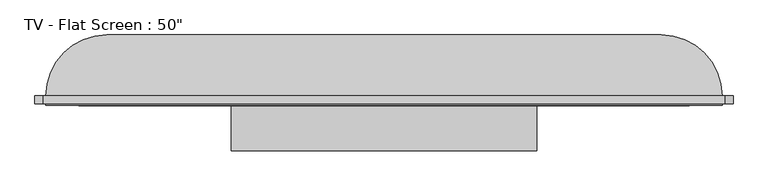
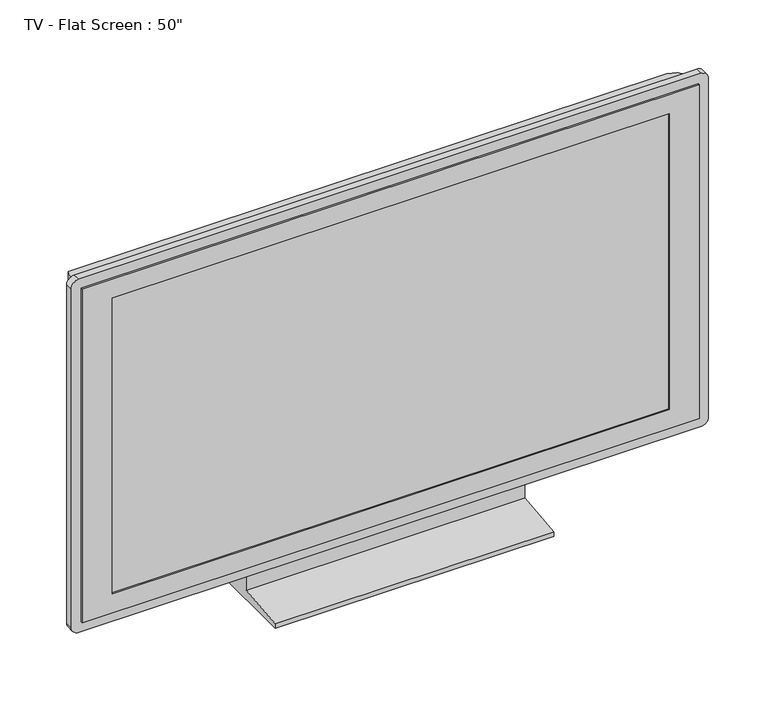
"""IFC4 building model written with IfcOpenShell, lengths in millimetres: furniture geometry."""

from ifc_helpers import new_model, si_unit, point, frame, frame_2d, origin, place, context, project, spatial, polyline, circle_curve, ellipse_curve, trimmed, segment, composite_curve, outline, extrude, faceted_brep, source, transform, mapped, element, save
from ifc_brep_helpers import plane_surface, cylinder_surface, advanced_brep


def furniture_0b81fedb(model_context):
    return source(origin(), model_context, "Body", "SolidModel", [
        advanced_brep(
        [(-617.3827737, -51.4613764, 80.0), (609.4937454, -51.4613764, 80.0), (609.4937454, -51.4613764, 782.6751733), (-617.3827737, -51.4613764, 782.6751733), (499.4937454, 58.5386236, 80.0), (-507.3827737, 58.5386236, 80.0), (-507.3827737, 58.5386236, 672.6751733), (499.4937454, 58.5386236, 672.6751733)],
        [
            (0, 1),
            (1, 2),
            (2, 3),
            (3, 0),
            (4, 5),
            (5, 6),
            (6, 7),
            (7, 4),
            (0, 5, circle_curve(frame((-507.3827737, -51.4613764, 80.0), z_axis=(0.0, 0.0, -1.0), x_axis=(-1.0, 0.0, 0.0)), 110.0)),
            (4, 1, circle_curve(frame((499.4937454, -51.4613764, 80.0), z_axis=(0.0, 0.0, -1.0), x_axis=(1.0, 0.0, 0.0)), 110.0)),
            (7, 2, ellipse_curve(frame((499.4937454, -51.4613764, 672.6751733), z_axis=(0.7071067811865475, 0.0, -0.7071067811865475), x_axis=(0.7071067811865474, 0.0, 0.7071067811865476)), 155.5634919, 110.0)),
            (6, 3, ellipse_curve(frame((-507.3827737, -51.4613764, 672.6751733), z_axis=(0.7071067811865475, 0.0, 0.7071067811865475), x_axis=(-0.7071067811865476, 0.0, 0.7071067811865474)), 155.5634919, 110.0)),
        ],
        [
            plane_surface(frame((-617.3827737, -51.4613764, 782.6751733), z_axis=(0.0, -1.0, 0.0), x_axis=(-1.0, 0.0, 0.0))),
            plane_surface(frame((-617.3827737, 58.5386236, 782.6751733), z_axis=(0.0, 1.0, 0.0), x_axis=(1.0, 0.0, 0.0))),
            plane_surface(frame((-617.3827737, -51.4613764, 80.0), z_axis=(0.0, 0.0, -1.0), x_axis=(0.0, 1.0, 0.0))),
            cylinder_surface(frame((499.4937454, -51.4613764, 80.0), z_axis=(0.0, 0.0, 1.0), x_axis=(1.0, 0.0, 0.0)), 110.0),
            cylinder_surface(frame((609.4937454, -51.4613764, 672.6751733), z_axis=(-1.0, 0.0, 0.0), x_axis=(0.0, 0.0, 1.0)), 110.0),
            cylinder_surface(frame((-507.3827737, -51.4613764, 782.6751733), z_axis=(0.0, 0.0, -1.0), x_axis=(-1.0, 0.0, 0.0)), 110.0),
        ],
        [
            (0, [[1, 2, 3, 4]]),
            (1, [[5, 6, 7, 8]]),
            (2, [[-1, 9, -5, 10]]),
            (3, [[11, -2, -10, -8]]),
            (4, [[-11, -7, 12, -3]]),
            (5, [[-12, -6, -9, -4]]),
        ],
    ),
        extrude(outline(composite_curve([segment(polyline([(802.6751733, 614.4937454), (802.6751733, -622.3827737)]), True, "CONTINUOUS"), segment(trimmed(circle_curve(frame_2d((787.6751733, -622.3827737)), 15.0), [point((802.6751733, -622.3827737))], [point((787.6751733, -637.3827737))], False, "CARTESIAN"), True, "CONTINUOUS"), segment(polyline([(787.6751733, -637.3827737), (75.0, -637.3827737)]), True, "CONTINUOUS"), segment(trimmed(circle_curve(frame_2d((75.0, -622.3827737)), 15.0), [point((75.0, -637.3827737))], [point((60.0, -622.3827737))], False, "CARTESIAN"), True, "CONTINUOUS"), segment(polyline([(60.0, -622.3827737), (60.0, 614.4937454)]), True, "CONTINUOUS"), segment(trimmed(circle_curve(frame_2d((75.0, 614.4937454)), 15.0), [point((60.0, 614.4937454))], [point((75.0, 629.4937454))], False, "CARTESIAN"), True, "CONTINUOUS"), segment(polyline([(75.0, 629.4937454), (787.6751733, 629.4937454)]), True, "CONTINUOUS"), segment(trimmed(circle_curve(frame_2d((787.6751733, 614.4937454)), 15.0), [point((787.6751733, 629.4937454))], [point((802.6751733, 614.4937454))], False, "CARTESIAN"), True, "CONTINUOUS")], self_intersect=False), holes=[polyline([(782.6751733, 609.4937454), (80.0, 609.4937454), (80.0, -617.3827737), (782.6751733, -617.3827737), (782.6751733, 609.4937454)])]), frame((0.0, -66.4613764, 0.0), z_axis=(0.0, 1.0, 0.0), x_axis=(0.0, 0.0, 1.0)), (0.0, 0.0, 1.0), 15.0),
        faceted_brep([(609.4937454, -69.4613764, 782.6751733), (-617.3827737, -69.4613764, 782.6751733), (-617.3827737, -69.4613764, 80.0), (609.4937454, -69.4613764, 80.0), (-557.3827737, -69.4613764, 742.6751733), (549.4937454, -69.4613764, 742.6751733), (549.4937454, -69.4613764, 120.0), (-557.3827737, -69.4613764, 120.0), (609.4937454, -51.4613764, 782.6751733), (609.4937454, -51.4613764, 80.0), (-617.3827737, -51.4613764, 80.0), (-617.3827737, -51.4613764, 782.6751733), (-557.3827737, -66.4613764, 742.6751733), (-557.3827737, -66.4613764, 120.0), (549.4937454, -66.4613764, 120.0), (549.4937454, -66.4613764, 742.6751733)], [[[0, 1, 2, 3], [4, 5, 6, 7]], [[8, 9, 10, 11]], [[1, 0, 8, 11]], [[2, 1, 11, 10]], [[3, 2, 10, 9]], [[0, 3, 9, 8]], [[12, 13, 14, 15]], [[12, 15, 5, 4]], [[15, 14, 6, 5]], [[14, 13, 7, 6]], [[13, 12, 4, 7]]]),
        extrude(outline(polyline([(-51.4613764, 80.0), (-1.4613764, 80.0), (48.5386236, 0.0), (-151.4613764, 0.0), (-151.4613764, 10.0), (-51.4613764, 20.0), (-51.4613764, 80.0)])), frame((-280.6636439, 0.0, 0.0), z_axis=(1.0, 0.0, 0.0), x_axis=(0.0, 1.0, 0.0)), (0.0, 0.0, 1.0), 553.4382596),
    ])


if __name__ == "__main__":
    model = new_model("IFC4")
    model_context = context("Model", 3, world=origin())
    ifc_project = project(units=[si_unit("LENGTHUNIT", "METRE", prefix="MILLI")], contexts=[model_context])
    site = spatial("IfcSite", under=ifc_project)
    building = spatial("IfcBuilding", under=site)
    placement = place(None, origin())
    furniture_shape = furniture_0b81fedb(model_context)
    element("IfcFurniture", 1, ObjectType="TV - Flat Screen : 50\"", at=placement, inside=building, context=model_context, shape_type="MappedRepresentation", body=[
        mapped(furniture_shape, transform((0.0, 0.0, 0.0), x_axis=(1.0, 0.0, 0.0), y_axis=(0.0, 1.0, 0.0), z_axis=(0.0, 0.0, 1.0))),
    ])
    save(model, "model.ifc")

# Revit data of these elements
# Type "TV - Flat Screen : 50\""
#   SinAng = 0.001609 ft
#   L = 3.631485 ft
#   H = 2.042898 ft
#   Thickness = 0.360892 ft
#   Diagonal = 4.166667 ft
#   CosAng = 0.002859 ft
#   Stand [instance default] = yes
#   Default Elevation = 0
# Element 1 (IfcFurniture, "TV - Flat Screen : 50\"")
#   Materials on its faces: "TV - Black", "TV - Glass", "TV - Screen"
# Materials
#   "TV - Black": colour RGB 49 49 49, transparency 0
#   "TV - Glass": colour RGB 157 157 157, transparency 0.9
#   "TV - Screen": colour RGB 0 0 0, transparency 0
